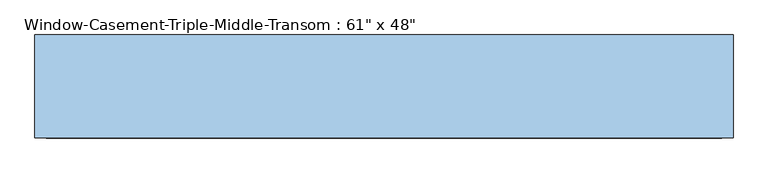
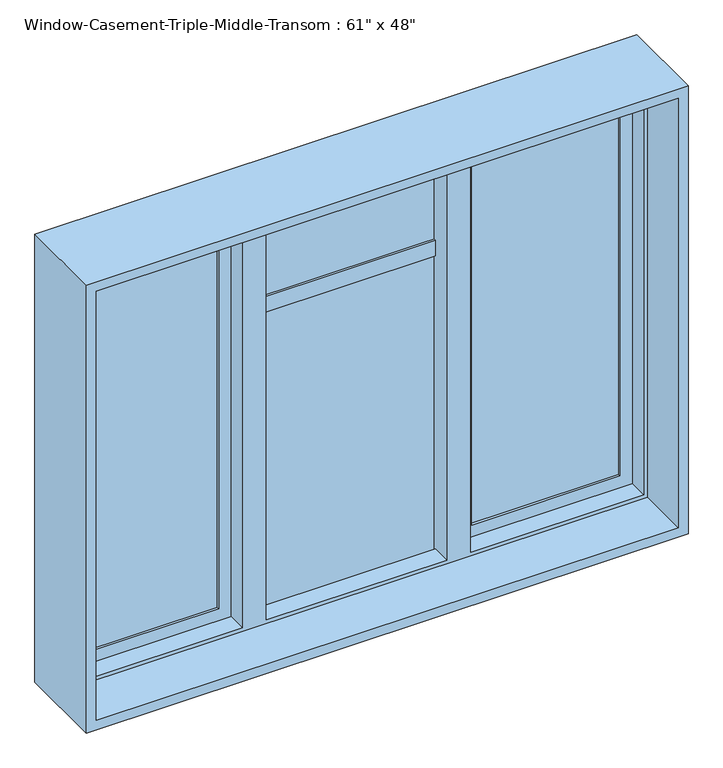
"""IFC4 building model written with IfcOpenShell, lengths in millimetres: window geometry."""

from ifc_helpers import new_model, si_unit, frame, origin, place, context, project, spatial, polyline, outline, extrude, faceted_brep, source, transform, mapped, element, save


def window_8c4be023(model_context):
    return source(origin(), model_context, "Body", "SolidModel", [
        extrude(outline(polyline([(2108.2, 283.6333333), (939.8, 283.6333333), (939.8, 749.3), (2108.2, 749.3), (2108.2, 283.6333333)]), holes=[polyline([(2066.3296875, 707.4296875), (981.6703125, 707.4296875), (981.6703125, 325.5036458), (2066.3296875, 325.5036458), (2066.3296875, 707.4296875)])]), frame((0.0, 73.025, 0.0), z_axis=(0.0, 1.0, 0.0), x_axis=(0.0, 0.0, 1.0)), (0.0, 0.0, 1.0), 31.75),
        extrude(outline(polyline([(2108.2, -749.3), (939.8, -749.3), (939.8, -283.6333333), (2108.2, -283.6333333), (2108.2, -749.3)]), holes=[polyline([(2066.3296875, -325.5036458), (981.6703125, -325.5036458), (981.6703125, -707.4296875), (2066.3296875, -707.4296875), (2066.3296875, -325.5036458)])]), frame((0.0, 73.025, 0.0), z_axis=(0.0, 1.0, 0.0), x_axis=(0.0, 0.0, 1.0)), (0.0, 0.0, 1.0), 31.75),
        extrude(outline(polyline([(-325.5036458, 98.425), (-325.5036458, 92.075), (-707.4296875, 92.075), (-707.4296875, 98.425), (-325.5036458, 98.425)])), frame((0.0, 0.0, 949.9203125), z_axis=(0.0, 0.0, 1.0), x_axis=(1.0, 0.0, 0.0)), (0.0, 0.0, 1.0), 1148.159375),
        extrude(outline(polyline([(-325.5036458, 85.725), (-325.5036458, 79.375), (-707.4296875, 79.375), (-707.4296875, 85.725), (-325.5036458, 85.725)])), frame((0.0, 0.0, 949.9203125), z_axis=(0.0, 0.0, 1.0), x_axis=(1.0, 0.0, 0.0)), (0.0, 0.0, 1.0), 1148.159375),
        extrude(outline(polyline([(707.4296875, 98.425), (707.4296875, 92.075), (325.5036458, 92.075), (325.5036458, 98.425), (707.4296875, 98.425)])), frame((0.0, 0.0, 949.9203125), z_axis=(0.0, 0.0, 1.0), x_axis=(1.0, 0.0, 0.0)), (0.0, 0.0, 1.0), 1148.159375),
        extrude(outline(polyline([(707.4296875, 85.725), (707.4296875, 79.375), (325.5036458, 79.375), (325.5036458, 85.725), (707.4296875, 85.725)])), frame((0.0, 0.0, 949.9203125), z_axis=(0.0, 0.0, 1.0), x_axis=(1.0, 0.0, 0.0)), (0.0, 0.0, 1.0), 1148.159375),
        extrude(outline(polyline([(232.8333333, 104.775), (232.8333333, 73.025), (-232.8333333, 73.025), (-232.8333333, 104.775), (232.8333333, 104.775)])), frame((0.0, 0.0, 1746.9048438), z_axis=(0.0, 0.0, 1.0), x_axis=(1.0, 0.0, 0.0)), (0.0, 0.0, 1.0), 41.8703125),
        extrude(outline(polyline([(232.8333333, 98.425), (232.8333333, 92.075), (-232.8333333, 92.075), (-232.8333333, 98.425), (232.8333333, 98.425)])), frame((0.0, 0.0, 939.8), z_axis=(0.0, 0.0, 1.0), x_axis=(1.0, 0.0, 0.0)), (0.0, 0.0, 1.0), 807.1048438),
        extrude(outline(polyline([(232.8333333, 85.725), (232.8333333, 79.375), (-232.8333333, 79.375), (-232.8333333, 85.725), (232.8333333, 85.725)])), frame((0.0, 0.0, 939.8), z_axis=(0.0, 0.0, 1.0), x_axis=(1.0, 0.0, 0.0)), (0.0, 0.0, 1.0), 807.1048438),
        extrude(outline(polyline([(232.8333333, 98.425), (232.8333333, 92.075), (-232.8333333, 92.075), (-232.8333333, 98.425), (232.8333333, 98.425)])), frame((0.0, 0.0, 1788.7751563), z_axis=(0.0, 0.0, 1.0), x_axis=(1.0, 0.0, 0.0)), (0.0, 0.0, 1.0), 319.4248438),
        extrude(outline(polyline([(232.8333333, 85.725), (232.8333333, 79.375), (-232.8333333, 79.375), (-232.8333333, 85.725), (232.8333333, 85.725)])), frame((0.0, 0.0, 1788.7751563), z_axis=(0.0, 0.0, 1.0), x_axis=(1.0, 0.0, 0.0)), (0.0, 0.0, 1.0), 319.4248438),
        faceted_brep([(-283.6333333, 73.025, 2108.2), (-749.3, 73.025, 2108.2), (-749.3, 114.3, 2108.2), (749.3, 114.3, 2108.2), (749.3, 73.025, 2108.2), (283.6333333, 73.025, 2108.2), (283.6333333, 111.125, 2108.2), (232.8333333, 111.125, 2108.2), (232.8333333, 73.025, 2108.2), (-232.8333333, 73.025, 2108.2), (-232.8333333, 111.125, 2108.2), (-283.6333333, 111.125, 2108.2), (-739.1796875, 22.225, 2098.0796875), (-739.1796875, 73.025, 2098.0796875), (-293.7536458, 73.025, 2098.0796875), (-293.7536458, 22.225, 2098.0796875), (739.1796875, 73.025, 2098.0796875), (739.1796875, 22.225, 2098.0796875), (293.7536458, 22.225, 2098.0796875), (293.7536458, 73.025, 2098.0796875), (-232.8333333, 73.025, 2098.0796875), (232.8333333, 73.025, 2098.0796875), (232.8333333, 22.225, 2098.0796875), (-232.8333333, 22.225, 2098.0796875), (-749.3, -114.3, 2108.2), (-749.3, 22.225, 2108.2), (749.3, 22.225, 2108.2), (749.3, -114.3, 2108.2), (-774.7, 114.3, 2133.6), (-774.7, -114.3, 2133.6), (774.7, -114.3, 2133.6), (774.7, 114.3, 2133.6), (749.3, 114.3, 939.8), (749.3, 73.025, 939.8), (739.1796875, 73.025, 949.9203125), (739.1796875, 22.225, 949.9203125), (749.3, 22.225, 939.8), (749.3, -114.3, 939.8), (774.7, -114.3, 914.4), (774.7, 114.3, 914.4), (283.6333333, 73.025, 939.8), (-749.3, 114.3, 939.8), (-749.3, 73.025, 939.8), (-283.6333333, 73.025, 939.8), (-283.6333333, 111.125, 939.8), (-232.8333333, 111.125, 939.8), (-232.8333333, 73.025, 939.8), (232.8333333, 73.025, 939.8), (232.8333333, 111.125, 939.8), (283.6333333, 111.125, 939.8), (293.7536458, 73.025, 949.9203125), (293.7536458, 22.225, 949.9203125), (-739.1796875, 73.025, 949.9203125), (-739.1796875, 22.225, 949.9203125), (-293.7536458, 22.225, 949.9203125), (-293.7536458, 73.025, 949.9203125), (232.8333333, 73.025, 949.9203125), (-232.8333333, 73.025, 949.9203125), (-232.8333333, 22.225, 949.9203125), (232.8333333, 22.225, 949.9203125), (-749.3, 22.225, 939.8), (-749.3, -114.3, 939.8), (-774.7, -114.3, 914.4), (-774.7, 114.3, 914.4)], [[[0, 1, 2, 3, 4, 5, 6, 7, 8, 9, 10, 11]], [[12, 13, 14, 15]], [[16, 17, 18, 19]], [[20, 21, 22, 23]], [[24, 25, 26, 27]], [[28, 29, 30, 31]], [[4, 3, 32, 33]], [[17, 16, 34, 35]], [[27, 26, 36, 37]], [[31, 30, 38, 39]], [[40, 33, 32, 41, 42, 43, 44, 45, 46, 47, 48, 49]], [[35, 34, 50, 51]], [[52, 53, 54, 55]], [[56, 57, 58, 59]], [[37, 36, 60, 61]], [[39, 38, 62, 63]], [[2, 1, 42, 41]], [[21, 20, 9, 8]], [[4, 33, 40, 5], [16, 19, 50, 34]], [[57, 56, 47, 46]], [[42, 1, 0, 43], [52, 55, 14, 13]], [[13, 12, 53, 52]], [[25, 24, 61, 60]], [[30, 29, 62, 38], [24, 27, 37, 61]], [[29, 28, 63, 62]], [[28, 31, 39, 63], [3, 2, 41, 32]], [[10, 45, 44, 11]], [[11, 44, 43, 0]], [[45, 10, 9, 20, 23, 58, 57, 46]], [[6, 49, 48, 7]], [[7, 48, 47, 56, 59, 22, 21, 8]], [[49, 6, 5, 40]], [[14, 55, 54, 15]], [[50, 19, 18, 51]], [[36, 26, 25, 60], [12, 15, 54, 53], [23, 22, 59, 58], [17, 35, 51, 18]]]),
    ])


if __name__ == "__main__":
    model = new_model("IFC4")
    model_context = context("Model", 3, world=origin())
    ifc_project = project(units=[si_unit("LENGTHUNIT", "METRE", prefix="MILLI")], contexts=[model_context])
    site = spatial("IfcSite", under=ifc_project)
    building = spatial("IfcBuilding", under=site)
    placement = place(None, origin())
    window_shape = window_8c4be023(model_context)
    element("IfcWindow", 1, ObjectType="Window-Casement-Triple-Middle-Transom : 61\" x 48\"", at=placement, inside=building, context=model_context, shape_type="MappedRepresentation", body=[
        mapped(window_shape, transform((0.0, 0.0, 0.0), x_axis=(1.0, 0.0, 0.0), y_axis=(0.0, 1.0, 0.0), z_axis=(0.0, 0.0, 1.0))),
    ])
    save(model, "model.ifc")

# Revit data of these elements
# Type "Window-Casement-Triple-Middle-Transom : 61\" x 48\""
#   Type Mark = "19"
#   Fire Rating = "0.5h"
#   Assembly Code = "B2020100"
#   Analytic Construction = "Double glazing - domestic"
#   Window Width = 1' - 8.33333"
#   Window Inset [instance default] = 0' - 0 5/8"
#   Wall Thickness [instance default] = 0' - 6"
#   Visual Light Transmittance = 0.81
#   Transom Height Ratio = 0.3
#   Thermal Resistance (R) = 1.8146 (h·ft²·°F)/BTU
#   Solar Heat Gain Coefficient = 0.76
#   Rough Width = 5' - 1 1/2"
#   Rough Height = 4' - 0 1/2"
#   Heat Transfer Coefficient (U) = 0.5511 BTU/(h·ft²·°F)
#   Height = 4' - 0"
#   Transom Height = 1' - 2.4"
#   Frame Gap 3 [instance default] = 0' - 1 83/128"
#   Frame Gap 2 [instance default] = 0' - 0 5/8"
#   Frame Gap 1 = 0' - 1 51/128"
#   Default Sill Height = 3' - 0"
#   Width = 5' - 1"
#   Frame Material = Metal - Aluminum
#   Glass Panel Material = Glass
#   Wall Closure = (empty or 0)
# Element 1 (IfcWindow, "Window-Casement-Triple-Middle-Transom : 61\" x 48\"")
#   Wall Thickness = 0' - 9"
#   Materials on its faces: "Metal - Aluminum", "Glass"
# Materials
#   "Metal - Aluminum": class "Metal", colour RGB 247 247 247, transparency 0
#   "Glass": class "Glass", colour RGB 0 128 192, transparency 0.75, Description = "Soda Lime Glass", Cost = 0
